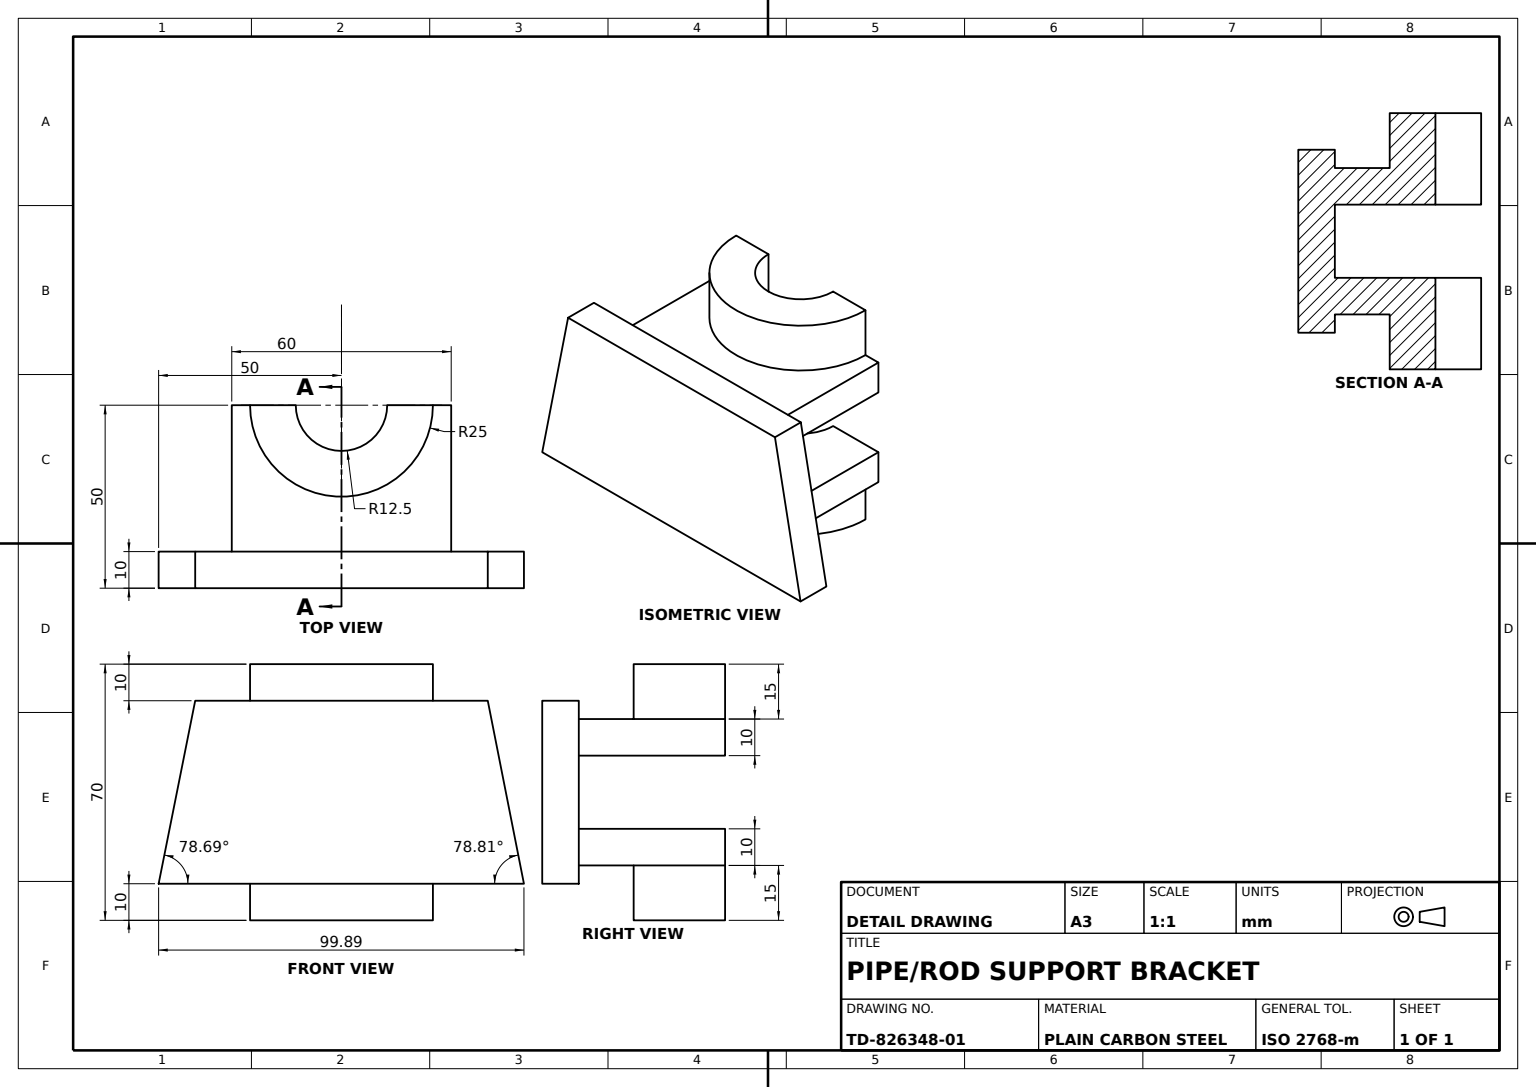
from build123d import *

# Parameters (mm, degrees)
BASE_PLATE_SKETCH_W          = 100
BASE_PLATE_SKETCH_H          = 50
BASE_PLATE_10MM_DEPTH        = 10
SUPPORT_ARM_DEPTH            = 10
ARM_RELIEF_CUT_SKETCH_R      = 12.5
ARM_RELIEF_CUT_DEPTH         = 117.726175299
BEARING_START                = 15
BEARING_SEAT_BOSS_15MM_DEPTH = 15
PLATE_TAPER_CUT_DEPTH        = 15


with BuildPart() as part:
    # Base Plate Sketch → Base Plate 10mm (new body)
    with BuildSketch(Plane.XY):
        with Locations((50, 25)):
            Rectangle(BASE_PLATE_SKETCH_W, BASE_PLATE_SKETCH_H)
    extrude(amount=BASE_PLATE_10MM_DEPTH)

    # Support Arm Sketch → Support Arm (add)
    with BuildSketch(Plane(origin=(0, 45, 0), x_dir=(1, 0, 0), z_dir=(0, 1, 0))):
        Polygon((50, 0), (20, 0), (20, 40), (80, 40), (80, 0), align=None)
    support_arm = extrude(amount=-SUPPORT_ARM_DEPTH)

    # Support Arm Mirror: Support Arm across plane
    add(support_arm.mirror(Plane.ZX.offset(25)))

    # Arm Relief Cut Sketch → Arm Relief Cut (cut, through all)
    with BuildSketch(Plane(origin=(0, 45, 0), x_dir=(1, 0, 0), z_dir=(0, 1, 0))):
        with Locations((50, 40)):
            Circle(ARM_RELIEF_CUT_SKETCH_R)
    extrude(amount=-ARM_RELIEF_CUT_DEPTH, mode=Mode.SUBTRACT)

    # Bearing Seat Boss Sketch → Bearing Seat Boss 15mm (add)
    with BuildSketch(Plane(origin=(0, 45, 0), x_dir=(1, 0, 0), z_dir=(0, 1, 0)).offset(BEARING_START)):
        with BuildLine():
            Line((25, 40), (37.5, 40))
            ThreePointArc((37.5, 40), (50, 27.5), (62.5, 40))
            Line((62.5, 40), (75, 40))
            ThreePointArc((75, 40), (50, 15), (25, 40))
        make_face()
    bearing_seat_boss_15mm = extrude(amount=-BEARING_SEAT_BOSS_15MM_DEPTH)

    # Bearing Seat Boss Mirror: Bearing Seat Boss 15mm across plane
    add(bearing_seat_boss_15mm.mirror(Plane.ZX.offset(25)))

    # Plate Taper Cut Sketch → Plate Taper Cut (cut)
    with BuildSketch(Plane(origin=(0, 0, 0), x_dir=(-1, 0, 0), z_dir=(0, 0, -1))):
        Polygon((-100, 50), (-90, 50), (-100, -0.55290415), align=None)
        Polygon((0, 50), (-10, 50), (0, 0), align=None)
    extrude(amount=-PLATE_TAPER_CUT_DEPTH, mode=Mode.SUBTRACT)


solid = part.part
